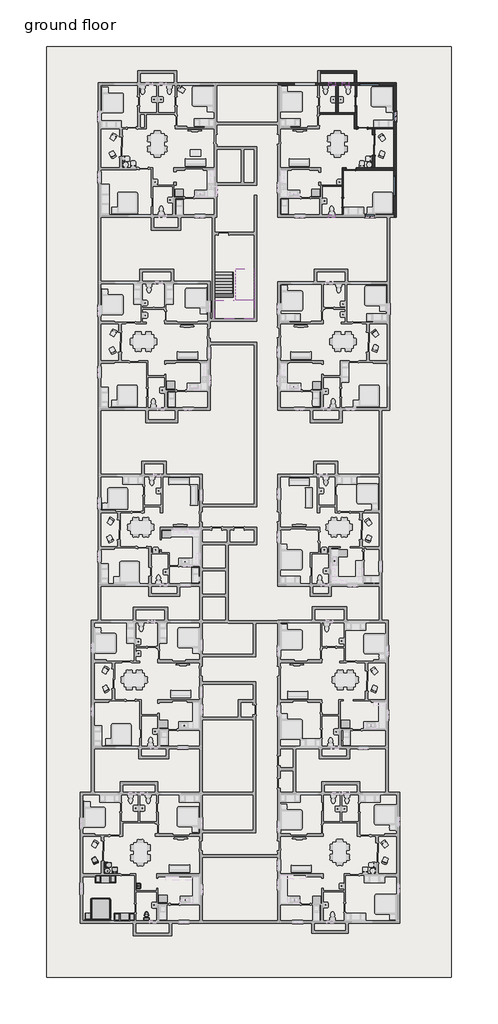
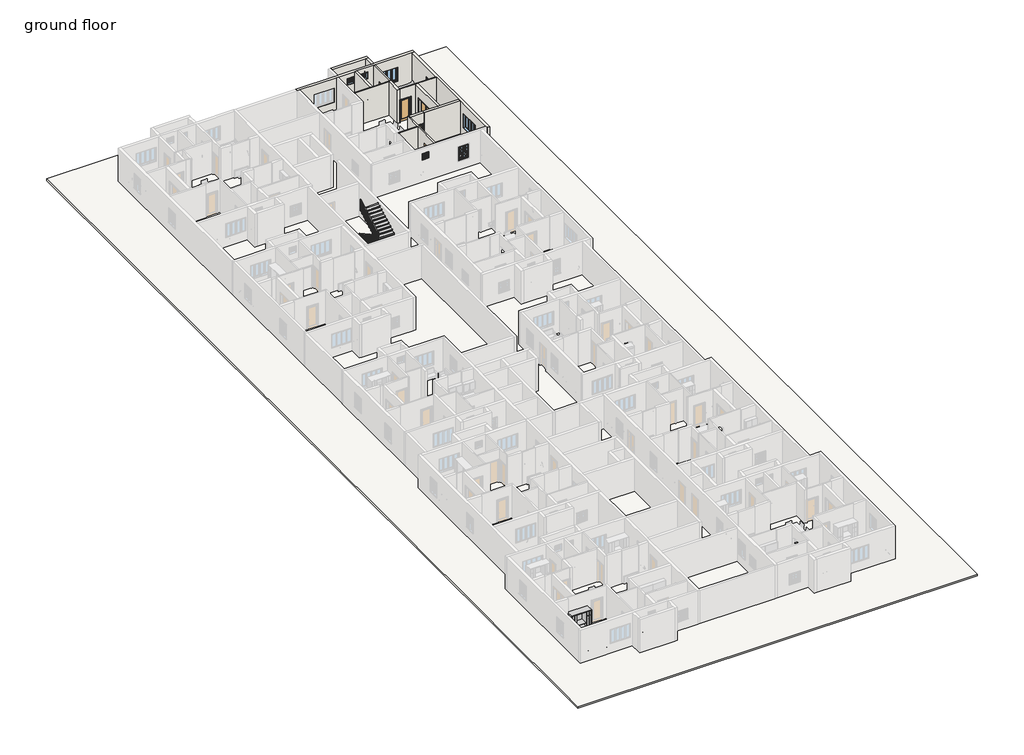
# One storey, part 10 of 16: 15 walls, 7 furniture elements, 7 windows, 5 doors, 2 flow terminals, 2 slabs, 2 stair flights, 1 railing.
# Revit data of these elements (continued)
# Element 6 (IfcFlowTerminal, "Sink Vanity-Square : 20\" x 18\"") (continued)
#   Materials on its faces: "Porcelain, Linen", "Steel, Polished"
# Element 7 (IfcFlowTerminal, "Toilet-Domestic-3D : Toilet-Domestic-3D")
#   Mark = "26"
#   Phase Created = New Construction
#   Materials on its faces: "Porcelain, Linen", "Laminate, Linen, Matte"
# Element 8 (IfcFurniture, "BED_DESIGN_8999 : BED_DESIGN_8999")
#   Phase Created = New Construction
#   Materials on its faces: "wood 2", "ss", "new wood", "fabric 2", "wood light", "fabric"
# Elements 9, 10 (IfcFurniture, "Entertainment Center : 72\" x 72\" x 24\"")
#   Phase Created = New Construction
#   Materials on its faces: "Steel, Chrome Plated", "Glass - Clear, Grey"
# Elements 11, 12, 13 (IfcFurniture, "Seating-Auditorium : 18\" x 24\" x 30\"")
#   Phase Created = New Construction
#   Materials on its faces: "Steel, Paint Finish, Dark Gray, Matte", "Linen, Beige"
# Element 14 (IfcFurniture, "Table-Trio End : 20\" Diameter")
#   Phase Created = New Construction
#   Materials on its faces: "Wood - Birch", "Laminate - Ivory,Matte"
# Element 15 (IfcRailing, "Handrail - Rectangular")
#   Phase Created = New Construction
# Element 16 (IfcSlab, "Generic - 6\"")
#   Height Offset From Level = -0' - 6"
#   Phase Created = New Construction
#   Materials on its faces: "Default Floor"
# Element 17 (IfcSlab, "Non-Monolithic Landing")
#   Phase Created = New Construction
# Elements 18, 19 (IfcStairFlight, "2\" Tread 1\" Nosing 1/4\" Riser")
#   Phase Created = New Construction
# Elements 20, 21, 22, 23 (IfcWall, "Generic - 4.5\"")
#   Top Offset = 0' - 0"
#   Base Offset = 0' - 0"
#   wall height = 10' - 6"
#   Phase Created = New Construction
#   Base Constraint = ground floor
#   Top Constraint = 1st floor
#   Materials on its faces: "Default Wall"
# Element 24 (IfcWall, "Generic - 6\"")
#   Top Offset = 0' - 0"
#   Base Offset = 0' - 0"
#   wall height = 10' - 6"
#   Phase Created = New Construction
#   Base Constraint = ground floor
#   Top Constraint = 1st floor
#   Materials on its faces: "Default Wall"
# Elements 25, 26, 27 (IfcWall, "Generic - 8\"")
#   Top Offset = 0' - 0"
#   Base Offset = 0' - 0"
#   wall height = 10' - 6"
#   Phase Created = New Construction
#   Base Constraint = ground floor
#   Top Constraint = 1st floor
#   Materials on its faces: "Default Wall"
# Elements 28, 29, 30, 31, 32, 33, 34 (IfcWall, "Generic - 9\"")
#   Top Offset = 0' - 0"
#   Base Offset = 0' - 0"
#   wall height = 10' - 6"
#   Phase Created = New Construction
#   Base Constraint = ground floor
#   Top Constraint = 1st floor
#   Materials on its faces: "Default Wall"
# Element 35 (IfcWindow, "Window-Casement-Multi-Sash-Horizontal : 72\" x 53\"")
#   Mark = "18"
#   Window Inset = 0' - 0 5/8"
#   Frame Gap 3 = 0' - 1 83/128"
#   Frame Gap 2 = 0' - 0 5/8"
#   Phase Created = New Construction
#   Materials on its faces: "Metal - Aluminum", "Glass"
# Element 36 (IfcWindow, "Window-Casement-Multi-Sash-Horizontal : 72\" x 53\"")
#   Mark = "19"
#   Window Inset = 0' - 0 5/8"
#   Frame Gap 3 = 0' - 1 83/128"
#   Frame Gap 2 = 0' - 0 5/8"
#   Phase Created = New Construction
#   Materials on its faces: "Metal - Aluminum", "Glass"
# Element 37 (IfcWindow, "Window-Louvers : 24\" x 24\"")
#   Mark = "91"
#   Blade Width = 1' - 10 1/2"
#   Phase Created = New Construction
#   Materials on its faces: "Birch"
# Element 38 (IfcWindow, "Window-Louvers : 24\" x 24\"")
#   Mark = "92"
#   Blade Width = 1' - 10 1/2"
#   Phase Created = New Construction
#   Materials on its faces: "Birch"
# Element 39 (IfcWindow, "Window-Louvers : 24\" x 24\"")
#   Mark = "93"
#   Blade Width = 1' - 10 1/2"
#   Phase Created = New Construction
#   Materials on its faces: "Birch"
# Element 40 (IfcWindow, "Window-Single-Hung-Double : 36\" x 52\"")
#   Mark = "43"
#   Window Inset = 0' - 0"
#   Interior Wall Closure = 0' - 1 1/2"
#   Frame Extension = 0' - 1 1/4"
#   Exterior Wall Closure = 0' - 0 1/2"
#   Interior Trim Visibility = yes
#   Indicator Visibility = yes
#   Exterior Trim Visibility = yes
#   Phase Created = New Construction
#   Materials on its faces: "Wood - Stained", "Glass", "Clad - White"
# Element 41 (IfcWindow, "Window-Single-Hung-Double : 36\" x 52\"")
#   Mark = "44"
#   Window Inset = 0' - 0"
#   Interior Wall Closure = 0' - 1 1/2"
#   Frame Extension = 0' - 1 1/4"
#   Exterior Wall Closure = 0' - 0 1/2"
#   Interior Trim Visibility = yes
#   Indicator Visibility = yes
#   Exterior Trim Visibility = yes
#   Phase Created = New Construction
#   Materials on its faces: "Wood - Stained", "Glass", "Clad - White"
# Materials
#   "Glass": class "Glass", colour RGB 0 128 192, transparency 0.75, Description = "Soda Lime Glass", Cost = 0
#   "Wood - Birch - Solid Stained Light Low Gloss": class "Wood", colour RGB 210 159 95, transparency 0, Cost = 0
#   "Paint - Sienna": colour RGB 118 70 51, transparency 0, Cost = 0
#   "Cherry": class "Wood", colour RGB 226 177 128, transparency 0, Description = "Prunus Serotina", Cost = 0
#   "Aluminum": class "Metal", colour RGB 247 247 247, transparency 0, Description = "Aluminum 6061", Cost = 0
#   "Door - Panel": class "Wood", colour RGB 210 159 95, transparency 0, Cost = 0
#   "Door - Frame": colour RGB 118 70 51, transparency 0, Cost = 0
#   "Porcelain, Linen": class "Ceramic", colour RGB 249 239 230, transparency 0, Description = "Porcelain, linen", Cost = 0
#   "Steel, Polished": class "Metal", colour RGB 192 192 192, transparency 0, Description = "Polished steel", Cost = 0
#   "Laminate, Linen, Matte": class "Plastic", colour RGB 249 239 230, transparency 0, Description = "Plastic Laminate - Linen, Matte", Cost = 0
#   "Linen, Beige": class "Textile", colour RGB 249 239 230, transparency 0, Description = "Linen, beige", Cost = 0
#   "Steel, Paint Finish, Dark Gray, Matte": class "Metal", colour RGB 0 0 0, transparency 0, Description = "Steel, paint finish, dark gray, matte", Cost = 0
#   "Wood - Birch": colour RGB 230 196 162, transparency 0
#   "Laminate - Ivory,Matte": colour RGB 127 127 127, transparency 0
#   "Metal - Aluminum": class "Metal", colour RGB 247 247 247, transparency 0
#   "Birch": class "Wood", colour RGB 224 178 126, transparency 0, Description = "Betula Alleghaniensis", Cost = 0
#   "Wood - Stained": class "Wood", colour RGB 224 178 126, transparency 0, Cost = 0
#   "Clad - White": class "Wood", colour RGB 242 242 238, transparency 0, Cost = 0
#   "wood 2": class "Wood", colour RGB 196 146 67, transparency 0
#   "ss": class "Metal", colour RGB 189 187 185, transparency 0
#   "new wood": class "Wood", colour RGB 133 62 31, transparency 0
#   "fabric 2": class "Fabric", colour RGB 198 193 133, transparency 0
#   "wood light": class "Wood", colour RGB 198 165 122, transparency 0
#   "fabric": class "Fabric", colour RGB 198 193 133, transparency 0
#   "Steel, Chrome Plated": class "Metal", colour RGB 17 17 17, transparency 0, Description = "Chromiuim plated steel", Cost = 0
#   "Glass - Clear, Grey": class "Glass", colour RGB 252 255 255, transparency 0.64
#   "Default Floor": colour RGB 128 128 128, transparency 0, Cost = 0
#   "Default Wall": colour RGB 128 128 128, transparency 0, Cost = 0
